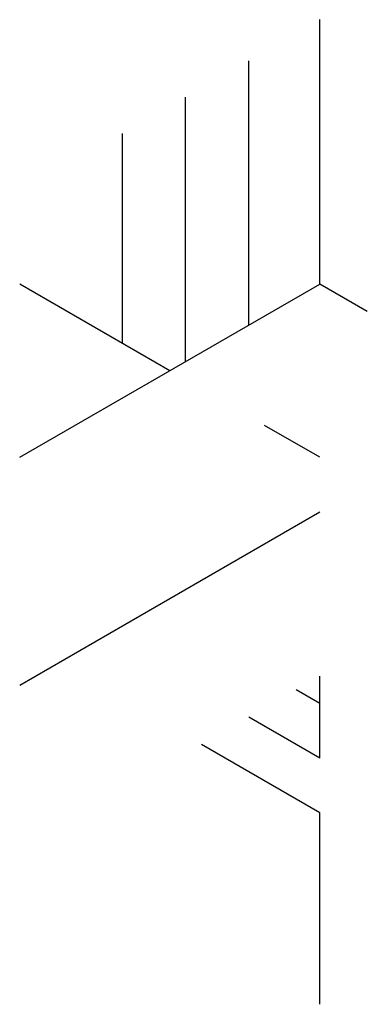
# Model space of a CAD drawing. Units: inches. Extents: x 5998 to 184806, y -27616 to 6737.
# Tile 3 of 3: x 179967 to 184806, y -27616 to -13900. Entities that reach past the tile are written whole.
import ezdxf

# ---------------------------------------------------------------- set-up
doc = ezdxf.new("R2010")
doc.units = ezdxf.units.IN
doc.header["$MEASUREMENT"] = 0
doc.layers.add('A-FURN', color=7, linetype='Continuous', lineweight=25)

msp = doc.modelspace()

# ---------------------------------------------------------------- linework, layer by layer
at = {"layer": 'A-FURN'}
for p, q in [((184147, -17583), (184147, -13900)), ((183157, -18155), (183157, -14472)), ((182277, -18663), (182277, -14980)), ((181397, -18409), (181397, -15488)), ((182057, -18790), (179967, -17583)), ((179967, -19996), (184147, -17583)), ((184806, -17964), (184147, -17583)), ((184147, -19996), (183377, -19552)), ((179967, -23171), (184147, -20758)), ((184147, -24187), (184147, -23044)), ((184147, -23425), (183817, -23235)), ((184147, -24187), (183157, -23616)), ((184147, -24949), (182497, -23997)), ((184147, -27616), (184147, -24949))]:
    msp.add_line(p, q, dxfattribs=at)

doc.saveas('drawing.dxf')
